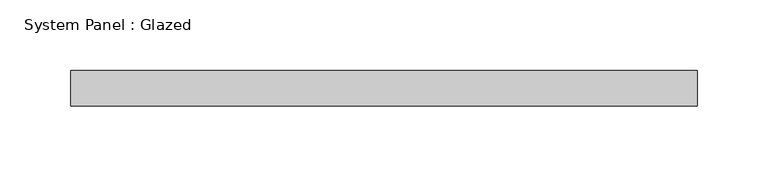
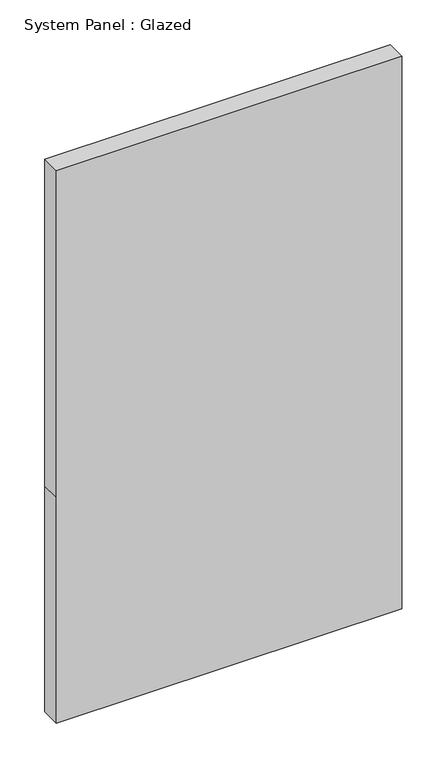
"""IFC4 building model written with IfcOpenShell, lengths in millimetres: plate geometry, System Panel : Glazed."""

from ifc_helpers import new_model, si_unit, frame, origin, place, context, project, spatial, polyline, outline, extrude, source, transform, mapped, element, save


def system_panel_glazed_00dbc574(model_context):
    return source(origin(), model_context, "Body", "SweptSolid", [
        extrude(outline(polyline([(0.0, -222.25), (0.0, 222.25), (306.9166667, 222.25), (751.4166667, 222.25), (751.4166667, -222.25), (306.9166667, -222.25), (0.0, -222.25)])), frame((0.0, 19.05, 0.0), z_axis=(0.0, 1.0, 0.0), x_axis=(0.0, 0.0, 1.0)), (0.0, 0.0, 1.0), 25.4),
    ])


if __name__ == "__main__":
    model = new_model("IFC4")
    model_context = context("Model", 3, world=origin())
    ifc_project = project(units=[si_unit("LENGTHUNIT", "METRE", prefix="MILLI")], contexts=[model_context])
    site = spatial("IfcSite", under=ifc_project)
    building = spatial("IfcBuilding", under=site)
    placement = place(None, origin())
    system_panel_glazed_shape = system_panel_glazed_00dbc574(model_context)
    element("IfcPlate", 1, ObjectType="System Panel : Glazed", at=placement, inside=building, context=model_context, shape_type="MappedRepresentation", body=[
        mapped(system_panel_glazed_shape, transform((0.0, 0.0, 0.0), x_axis=(1.0, 0.0, 0.0), y_axis=(0.0, 1.0, 0.0), z_axis=(0.0, 0.0, 1.0))),
    ])
    save(model, "model.ifc")

# Revit data of these elements
# Type "System Panel : Glazed"
#   Construction Type Id = "GSP4R"
#   Analytic Construction = "1/8 in Pilkington single glazing"
#   Visual Light Transmittance = 0.9
#   Solar Heat Gain Coefficient = 0.86
#   Heat Transfer Coefficient (U) = 1.18115 BTU/(h·ft²·°F)
#   Define Thermal Properties by = 1
# Element 1 (IfcPlate, "System Panel : Glazed")
#   Materials on its faces: "Glass"
# Materials
#   "Glass": class "Glass", colour RGB 0 128 192, transparency 0.75, Description = "Soda Lime Glass", Cost = 0
